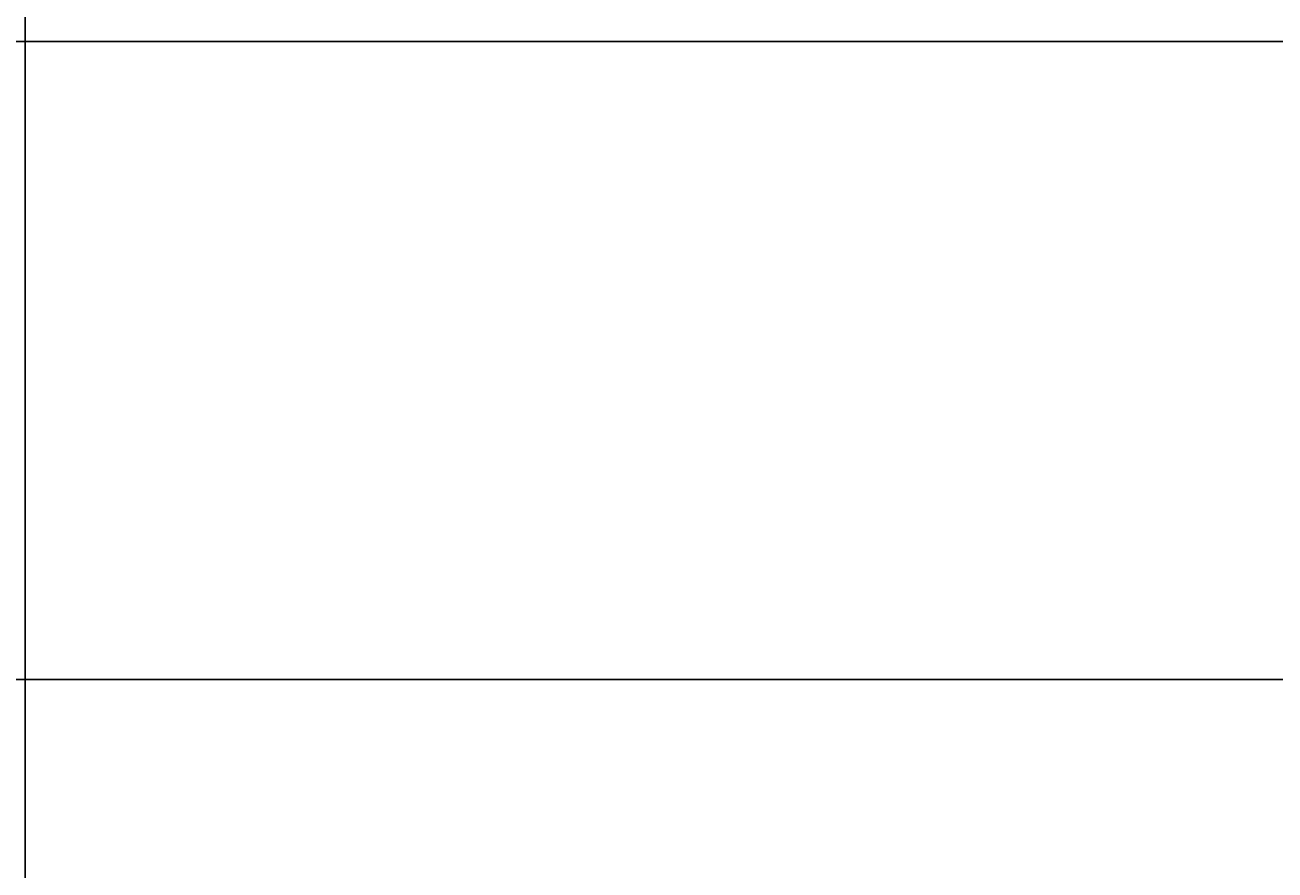
# Model space of a CAD drawing. Units: inches. Extents: x 35362 to 73946, y 43607 to 67532.
# Tile 134 of 134: x 67327 to 68296, y 55752 to 56407. Entities that reach past the tile are written whole.
import ezdxf

# ---------------------------------------------------------------- set-up
doc = ezdxf.new("R2010")
doc.units = ezdxf.units.IN
doc.header["$MEASUREMENT"] = 0
doc.layers.add('A-ANNO-DIMS', color=2, linetype='Continuous', lineweight=18)
doc.styles.get("Standard").update_dxf_attribs({"font": 'arial.ttf'})
doc.dimstyles.get("Standard").update_dxf_attribs({"dimtxt": 0.18, "dimasz": 0.18, "dimexe": 0.18, "dimexo": 0.0625, "dimgap": 0.09, "dimtad": 0, "dimtih": 1, "dimtoh": 1, "dimdec": 4, "dimzin": 0, "dimdsep": 46, "dimtxsty": 'Standard', "dimcen": 0.09, "dimadec": 0, "dimazin": 0, "dimtfac": 1, "dimtdec": 4, "dimtofl": 0, "dimtmove": 0, "dimatfit": 3, "dimfxl": 1, "dimtolj": 1, "dimtzin": 0, "dimarcsym": 0})

# ---------------------------------------------------------------- blocks, each defined once
blk = doc.blocks.new('*D8')
at = {"layer": 'A-ANNO-DIMS', "color": 0, "lineweight": -2, "transparency": 16777216}
for p, q in [((66271.28651900003, 65771.51172800003), (73945.82566600003, 65771.51172800003)), ((73945.64566600005, 65771.33172800003), (73945.64566600005, 59737.03093663782)), ((73945.64566600005, 53702.36633900002), (73945.64566600005, 59736.66713036224)), ((72185.70816600003, 53702.18633900003), (73945.82566600003, 53702.18633900003))]:
    blk.add_line(p, q, dxfattribs=at)
at = {"layer": 'A-ANNO-DIMS', "color": 0, "transparency": 16777216}
for points in [[(73945.61566600006, 65771.33172800003), (73945.67566600005, 65771.33172800003), (73945.64566600005, 65771.51172800003)], [(73945.61566600006, 53702.36633900002), (73945.67566600005, 53702.36633900002), (73945.64566600005, 53702.18633900003)]]:
    blk.add_solid(points, dxfattribs=at)
at = {"layer": 'Defpoints', "color": 0, "transparency": 16777216}
for p in [(66271.22401900003, 65771.51172800003), (73945.64566600005, 65771.51172800003), (72185.64566600003, 53702.18633900003)]:
    blk.add_point(p, dxfattribs=at)
at = {"layer": 'A-ANNO-DIMS', "color": 0, "transparency": 16777216, "insert": (73945.64566600005, 59736.84903349999), "char_height": 0.18, "attachment_point": 5}
blk.add_mtext('\\A1;12069', dxfattribs=at)
blk = doc.blocks.new('*D10')
at = {"layer": 'A-ANNO-DIMS', "color": 0, "lineweight": -2, "transparency": 16777216}
for p, q in [((61240.96983600002, 59185.14395700003), (73945.82566600003, 59185.14395700003)), ((73945.64566600005, 59184.96395700003), (73945.64566600005, 56268.51827402935)), ((73945.64566600005, 53351.70866200003), (73945.64566600005, 56268.1543449707)), ((61240.96983600002, 53351.52866200003), (73945.82566600003, 53351.52866200003))]:
    blk.add_line(p, q, dxfattribs=at)
at = {"layer": 'A-ANNO-DIMS', "color": 0, "transparency": 16777216}
for points in [[(73945.61566600006, 59184.96395700003), (73945.67566600005, 59184.96395700003), (73945.64566600005, 59185.14395700003)], [(73945.61566600006, 53351.70866200003), (73945.67566600005, 53351.70866200003), (73945.64566600005, 53351.52866200003)]]:
    blk.add_solid(points, dxfattribs=at)
at = {"layer": 'Defpoints', "color": 0, "transparency": 16777216}
for p in [(61240.90733600002, 59185.14395700003), (61240.90733600002, 53351.52866200003), (73945.64566600005, 53351.52866200003)]:
    blk.add_point(p, dxfattribs=at)
at = {"layer": 'A-ANNO-DIMS', "color": 0, "transparency": 16777216, "insert": (73945.64566600005, 56268.33630949999), "char_height": 0.18, "attachment_point": 5}
blk.add_mtext('\\A1;5834', dxfattribs=at)
blk = doc.blocks.new('*D36')
at = {"layer": 'A-ANNO-DIMS', "color": 0, "lineweight": -2, "transparency": 16777216}
for p, q in [((68320.80826200004, 60122.34633200002), (35361.76908500003, 60122.34633200002)), ((35361.94908500003, 60122.16633200002), (35361.94908500003, 57247.82893113781)), ((35361.94908500003, 54373.12772400002), (35361.94908500003, 57247.46512486223)), ((68320.80826200004, 54372.94772400003), (35361.76908500003, 54372.94772400002))]:
    blk.add_line(p, q, dxfattribs=at)
at = {"layer": 'A-ANNO-DIMS', "color": 0, "transparency": 16777216}
for points in [[(35361.91908500003, 60122.16633200002), (35361.97908500003, 60122.16633200002), (35361.94908500003, 60122.34633200002)], [(35361.91908500003, 54373.12772400002), (35361.97908500003, 54373.12772400002), (35361.94908500003, 54372.94772400002)]]:
    blk.add_solid(points, dxfattribs=at)
at = {"layer": 'Defpoints', "color": 0, "transparency": 16777216}
for p in [(68320.87076200004, 60122.34633200002), (35361.94908500003, 54372.94772400002), (68320.87076200004, 54372.94772400003)]:
    blk.add_point(p, dxfattribs=at)
at = {"layer": 'A-ANNO-DIMS', "color": 0, "transparency": 16777216, "insert": (35361.94908500004, 57247.64702799999), "char_height": 0.18, "attachment_point": 5}
blk.add_mtext('\\A1;5749.4', dxfattribs=at)
blk = doc.blocks.new('*D50')
at = {"layer": 'A-ANNO-DIMS', "color": 0, "lineweight": -2, "transparency": 16777216}
for p, q in [((61657.28213900003, 56394.41825000003), (73945.82566600003, 56394.41825000003)), ((73945.64566600005, 56394.23825000003), (73945.64566600005, 56147.19337413782)), ((73945.64566600005, 55899.78469200003), (73945.64566600005, 56146.82956786224)), ((61657.28213900003, 55899.60469200002), (73945.82566600003, 55899.60469200002))]:
    blk.add_line(p, q, dxfattribs=at)
at = {"layer": 'A-ANNO-DIMS', "color": 0, "transparency": 16777216}
for points in [[(73945.61566600006, 56394.23825000003), (73945.67566600005, 56394.23825000003), (73945.64566600005, 56394.41825000003)], [(73945.61566600006, 55899.78469200003), (73945.67566600005, 55899.78469200003), (73945.64566600005, 55899.60469200002)]]:
    blk.add_solid(points, dxfattribs=at)
at = {"layer": 'Defpoints', "color": 0, "transparency": 16777216}
for p in [(61657.21963900003, 56394.41825000003), (61657.21963900003, 55899.60469200002), (73945.64566600005, 55899.60469200002)]:
    blk.add_point(p, dxfattribs=at)
at = {"layer": 'A-ANNO-DIMS', "color": 0, "transparency": 16777216, "insert": (73945.64566600005, 56147.01147099999), "char_height": 0.18, "attachment_point": 5}
blk.add_mtext('\\A1;494.8', dxfattribs=at)
blk = doc.blocks.new('*D65')
at = {"layer": 'A-ANNO-DIMS', "color": 0, "lineweight": -2, "transparency": 16777216}
for p, q in [((65336.01600799999, 61293.223552), (65336.01600799999, 43606.678996)), ((67326.639741, 61293.223552), (67326.639741, 43606.678996)), ((65336.19600799999, 43606.858996), (66330.87277900206, 43606.858996)), ((67326.45974100001, 43606.858996), (66331.78296999796, 43606.858996))]:
    blk.add_line(p, q, dxfattribs=at)
at = {"layer": 'A-ANNO-DIMS', "color": 0, "transparency": 16777216}
for points in [[(65336.19600799999, 43606.888996), (65336.19600799999, 43606.828996), (65336.01600799999, 43606.858996)], [(67326.45974100001, 43606.888996), (67326.45974100001, 43606.828996), (67326.639741, 43606.858996)]]:
    blk.add_solid(points, dxfattribs=at)
at = {"layer": 'Defpoints', "color": 0, "transparency": 16777216}
for p in [(65336.01600799999, 61293.286052), (67326.639741, 61293.286052), (67326.639741, 43606.858996)]:
    blk.add_point(p, dxfattribs=at)
at = {"layer": 'A-ANNO-DIMS', "color": 0, "transparency": 16777216, "insert": (66331.32787450001, 43606.858996), "char_height": 0.18, "attachment_point": 5}
blk.add_mtext('\\A1;1990.6', dxfattribs=at)

msp = doc.modelspace()

# ---------------------------------------------------------------- dimensions: what is measured, and where the dimension line sits
at = {"layer": 'A-ANNO-DIMS'}
for base, p1, p2, override, picture, middle in [((73945.64566600005, 65771.51172800003), (72185.645666, 53702.186339), (66271.224019, 65771.51172799998), {"dimdec": 0, "dimlfac": 1, "dimrnd": 0, "dimzin": 0, "dimdsep": 46, "dimlunit": 2}, '*D8', (73945.64566600005, 59736.84903349999)), ((35361.94908500003, 54372.94772400002), (68320.870762, 60122.346332), (68320.870762, 54372.947724), {"dimdec": 1, "dimlfac": 1, "dimrnd": 0, "dimzin": 0, "dimdsep": 46, "dimlunit": 2}, '*D36', (35361.94908500004, 57247.64702799999)), ((73945.64566600005, 53351.52866200003), (61240.907336, 59185.14395699999), (61240.907336, 53351.52866199999), {"dimdec": 0, "dimlfac": 1, "dimrnd": 0, "dimzin": 0, "dimdsep": 46, "dimlunit": 2}, '*D10', (73945.64566600005, 56268.33630949999)), ((73945.64566600005, 55899.60469200002), (61657.219639, 56394.41825), (61657.219639, 55899.604692), {"dimdec": 1, "dimlfac": 1, "dimrnd": 0, "dimzin": 0, "dimdsep": 46, "dimlunit": 2}, '*D50', (73945.64566600005, 56147.01147099999))]:
    dim = msp.add_linear_dim(base=base, p1=p1, p2=p2, angle=90, dimstyle='Standard', override=override, dxfattribs=at)
    dim.commit()
    dim.dimension.update_dxf_attribs({"geometry": picture, "text_midpoint": middle})
dim = msp.add_linear_dim(base=(67326.639741, 43606.858996), p1=(65336.01600799999, 61293.286052), p2=(67326.639741, 61293.286052), dimstyle='Standard', override={"dimdec": 1, "dimlfac": 1, "dimrnd": 0, "dimzin": 0, "dimdsep": 46, "dimlunit": 2}, dxfattribs=at)
dim.commit()
dim.dimension.update_dxf_attribs({"geometry": '*D65', "text_midpoint": (66331.32787450001, 43606.858996)})

doc.saveas('drawing.dxf')
